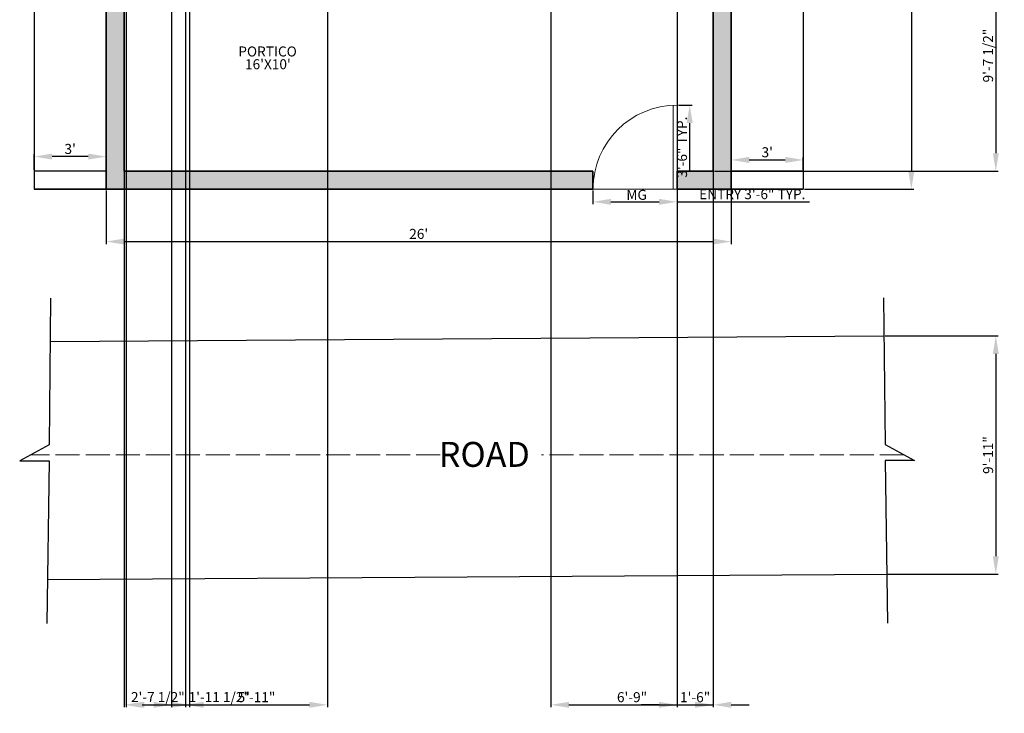
# Model space of a CAD drawing. Units: inches. Extents: x 2265 to 2807, y 1544 to 2401.
# Tile 1 of 9: x 2316 to 2807, y 1544 to 1890. Entities that reach past the tile are written whole.
import ezdxf

# ---------------------------------------------------------------- set-up
doc = ezdxf.new("R2010")
doc.units = ezdxf.units.IN
doc.linetypes.add('ACAD_ISO02W100', pattern=[15, 12, -3])
for name, color, linetype, lineweight in [('A-ANNO-DIMS', 2, 'Continuous', 18), ('A-ANNO-TEXT', 7, 'Continuous', 18), ('A-AREA-IDEN', 7, 'Continuous', 18), ('A-DOOR', 3, 'Continuous', 18), ('A-WALL', 7, 'Continuous', 35), ('A-WALL-PATT', 18, 'Continuous', 13), ('C-PROP', 7, 'Continuous', 25), ('C-ROAD', 8, 'Continuous', 25), ('C-ROAD-CNTR', 8, 'ACAD_ISO02W100', 18)]:
    doc.layers.add(name, color=color, linetype=linetype, lineweight=lineweight)
doc.styles.add('ARIAL', font='times.ttf', dxfattribs={"height": 5})
doc.styles.get("Standard").update_dxf_attribs({"font": 'arial.ttf', "height": 5})
doc.dimstyles.new('ISO-25', dxfattribs={"dimtxt": 5, "dimasz": 9, "dimexe": 1.25, "dimexo": 0.625, "dimtad": 1, "dimlunit": 3, "dimtxsty": 'Standard', "dimcen": 2.5, "dimadec": 0, "dimazin": 0, "dimtfac": 1, "dimtmove": 0, "dimatfit": 3, "dimfxl": 1, "dimarcsym": 0})

# ---------------------------------------------------------------- blocks, each defined once
blk = doc.blocks.new('*D2')
at = {"layer": 'A-ANNO-DIMS', "color": 0, "lineweight": -2, "transparency": 16777216}
for p, q in [((2323.1, 1815.36), (2323.1, 1823.27)), ((2350.1, 1822.02), (2332.1, 1822.02)), ((2359.1, 1815.36), (2359.1, 1823.27))]:
    blk.add_line(p, q, dxfattribs=at)
at = {"layer": 'A-ANNO-DIMS', "color": 0, "lineweight": 100, "transparency": 16777216}
for points in [[(2332.1, 1823.52), (2332.1, 1820.52), (2323.1, 1822.02)], [(2350.1, 1823.52), (2350.1, 1820.52), (2359.1, 1822.02)]]:
    blk.add_solid(points, dxfattribs=at)
at = {"layer": 'Defpoints', "color": 0, "lineweight": 100, "transparency": 16777216}
for p in [(2323.1, 1822.02), (2323.1, 1814.73), (2359.1, 1814.73)]:
    blk.add_point(p, dxfattribs=at)
at = {"layer": 'A-ANNO-DIMS', "color": 0, "transparency": 16777216, "insert": (2341.1, 1825.2), "char_height": 5, "attachment_point": 5}
blk.add_mtext("3'", dxfattribs=at)
blk = doc.blocks.new('*D3')
at = {"layer": 'A-ANNO-DIMS', "color": 0, "lineweight": -2, "transparency": 16777216}
for p, q in [((2671.1, 1815.36), (2671.1, 1821.61)), ((2680.1, 1820.36), (2698.1, 1820.36)), ((2707.1, 1815.36), (2707.1, 1821.61))]:
    blk.add_line(p, q, dxfattribs=at)
at = {"layer": 'A-ANNO-DIMS', "color": 0, "lineweight": 100, "transparency": 16777216}
for points in [[(2680.1, 1821.86), (2680.1, 1818.86), (2671.1, 1820.36)], [(2698.1, 1821.86), (2698.1, 1818.86), (2707.1, 1820.36)]]:
    blk.add_solid(points, dxfattribs=at)
at = {"layer": 'Defpoints', "color": 0, "lineweight": 100, "transparency": 16777216}
for p in [(2707.1, 1820.36), (2671.1, 1814.73), (2707.1, 1814.73)]:
    blk.add_point(p, dxfattribs=at)
at = {"layer": 'A-ANNO-DIMS', "color": 0, "transparency": 16777216, "insert": (2689.1, 1823.54), "char_height": 5, "attachment_point": 5}
blk.add_mtext("3'", dxfattribs=at)
blk = doc.blocks.new('*D4')
at = {"layer": 'A-ANNO-DIMS', "color": 0, "lineweight": -2, "transparency": 16777216}
for p, q in [((2359.1, 1805.11), (2359.1, 1778.33)), ((2671.1, 1805.11), (2671.1, 1778.33)), ((2368.1, 1779.58), (2662.1, 1779.58))]:
    blk.add_line(p, q, dxfattribs=at)
at = {"layer": 'A-ANNO-DIMS', "color": 0, "lineweight": 100, "transparency": 16777216}
for points in [[(2368.1, 1781.08), (2368.1, 1778.08), (2359.1, 1779.58)], [(2662.1, 1781.08), (2662.1, 1778.08), (2671.1, 1779.58)]]:
    blk.add_solid(points, dxfattribs=at)
at = {"layer": 'Defpoints', "color": 0, "lineweight": 100, "transparency": 16777216}
for p in [(2359.1, 1805.73), (2671.1, 1805.73), (2671.1, 1779.58)]:
    blk.add_point(p, dxfattribs=at)
at = {"layer": 'A-ANNO-DIMS', "color": 0, "transparency": 16777216, "insert": (2515.1, 1782.76), "char_height": 5, "attachment_point": 5}
blk.add_mtext("26'", dxfattribs=at)
blk = doc.blocks.new('*D6')
at = {"layer": 'A-ANNO-DIMS', "color": 0, "lineweight": -2, "transparency": 16777216}
for p, q in [((2707.73, 2255.73), (2762.29, 2255.73)), ((2761.04, 2246.73), (2761.04, 1814.73)), ((2707.73, 1805.73), (2762.29, 1805.73))]:
    blk.add_line(p, q, dxfattribs=at)
at = {"layer": 'A-ANNO-DIMS', "color": 0, "lineweight": 100, "transparency": 16777216}
for points in [[(2759.54, 2246.73), (2762.54, 2246.73), (2761.04, 2255.73)], [(2759.54, 1814.73), (2762.54, 1814.73), (2761.04, 1805.73)]]:
    blk.add_solid(points, dxfattribs=at)
at = {"layer": 'Defpoints', "color": 0, "lineweight": 100, "transparency": 16777216}
for p in [(2707.1, 2255.73), (2707.1, 1805.73), (2761.04, 1805.73)]:
    blk.add_point(p, dxfattribs=at)
at = {"layer": 'A-ANNO-DIMS', "color": 0, "transparency": 16777216, "insert": (2757.86, 2030.73), "char_height": 5, "attachment_point": 5, "rotation": 90}
blk.add_mtext('37\'-6"', dxfattribs=at)
blk = doc.blocks.new('ROAD-BREAK')
for p, q in [((15.45, 162.46), (14.64, 89.26)), ((14.64, 89.26), (0, 81.28)), ((0, 81.28), (14.64, 81.28)), ((14.64, 81.28), (13.51, 0))]:
    blk.add_line(p, q)
blk = doc.blocks.new('DOOR-SWING-42IN')
for p, q in [((40, 41.95), (40, 0)), ((42, 0), (0, 0))]:
    blk.add_line(p, q)
blk.add_arc((42, 0), 42, 90, 180)
blk = doc.blocks.new('*D25')
at = {"layer": 'A-ANNO-DIMS', "color": 0, "lineweight": -2, "transparency": 16777216}
for p, q in [((2602.1, 1805.11), (2602.1, 1798.18)), ((2644.1, 1805.11), (2644.1, 1798.18)), ((2611.1, 1799.43), (2635.1, 1799.43)), ((2644.1, 1799.43), (2710.18, 1799.43))]:
    blk.add_line(p, q, dxfattribs=at)
at = {"layer": 'A-ANNO-DIMS', "color": 0, "lineweight": 100, "transparency": 16777216}
for points in [[(2611.1, 1800.93), (2611.1, 1797.93), (2602.1, 1799.43)], [(2635.1, 1800.93), (2635.1, 1797.93), (2644.1, 1799.43)]]:
    blk.add_solid(points, dxfattribs=at)
at = {"layer": 'Defpoints', "color": 0, "lineweight": 100, "transparency": 16777216}
for p in [(2602.1, 1805.73), (2644.1, 1805.73), (2644.1, 1799.43)]:
    blk.add_point(p, dxfattribs=at)
at = {"layer": 'A-ANNO-DIMS', "color": 0, "transparency": 16777216, "insert": (2681.64, 1802.61), "char_height": 5, "attachment_point": 5}
blk.add_mtext('ENTRY 3\'-6" TYP.', dxfattribs=at)
blk = doc.blocks.new('*D26')
at = {"layer": 'A-ANNO-DIMS', "color": 0, "lineweight": -2, "transparency": 16777216}
for p, q in [((2644.73, 1847.73), (2651.65, 1847.73)), ((2650.4, 1814.73), (2650.4, 1838.73)), ((2644.73, 1805.73), (2651.65, 1805.73))]:
    blk.add_line(p, q, dxfattribs=at)
at = {"layer": 'A-ANNO-DIMS', "color": 0, "lineweight": 100, "transparency": 16777216}
for points in [[(2648.9, 1838.73), (2651.9, 1838.73), (2650.4, 1847.73)], [(2648.9, 1814.73), (2651.9, 1814.73), (2650.4, 1805.73)]]:
    blk.add_solid(points, dxfattribs=at)
at = {"layer": 'Defpoints', "color": 0, "lineweight": 100, "transparency": 16777216}
for p in [(2644.1, 1847.73), (2650.4, 1847.73), (2644.1, 1805.73)]:
    blk.add_point(p, dxfattribs=at)
at = {"layer": 'A-ANNO-DIMS', "color": 0, "transparency": 16777216, "insert": (2647.22, 1826.73), "char_height": 5, "attachment_point": 5, "rotation": 90}
blk.add_mtext('3\'-6" TYP.', dxfattribs=at)
blk = doc.blocks.new('*D35')
at = {"layer": 'A-ANNO-DIMS', "color": 0, "lineweight": -2, "transparency": 16777216}
for p, q in [((2581.1, 2123.11), (2581.1, 1546.93)), ((2662.1, 2123.11), (2662.1, 1546.93)), ((2590.1, 1548.18), (2653.1, 1548.18))]:
    blk.add_line(p, q, dxfattribs=at)
at = {"layer": 'A-ANNO-DIMS', "color": 0, "lineweight": 100, "transparency": 16777216}
for points in [[(2590.1, 1549.68), (2590.1, 1546.68), (2581.1, 1548.18)], [(2653.1, 1549.68), (2653.1, 1546.68), (2662.1, 1548.18)]]:
    blk.add_solid(points, dxfattribs=at)
at = {"layer": 'Defpoints', "color": 0, "lineweight": 100, "transparency": 16777216}
for p in [(2581.1, 2123.73), (2662.1, 2123.73), (2662.1, 1548.18)]:
    blk.add_point(p, dxfattribs=at)
at = {"layer": 'A-ANNO-DIMS', "color": 0, "transparency": 16777216, "insert": (2621.6, 1551.36), "char_height": 5, "attachment_point": 5}
blk.add_mtext('6\'-9"', dxfattribs=at)
blk = doc.blocks.new('*D38')
at = {"layer": 'A-ANNO-DIMS', "color": 0, "lineweight": -2, "transparency": 16777216}
for p, q in [((2747.98, 1732.42), (2804.46, 1732.42)), ((2803.21, 1723.42), (2803.21, 1622.43)), ((2749.38, 1613.43), (2804.46, 1613.43))]:
    blk.add_line(p, q, dxfattribs=at)
at = {"layer": 'A-ANNO-DIMS', "color": 0, "lineweight": 100, "transparency": 16777216}
for points in [[(2801.71, 1723.42), (2804.71, 1723.42), (2803.21, 1732.42)], [(2801.71, 1622.43), (2804.71, 1622.43), (2803.21, 1613.43)]]:
    blk.add_solid(points, dxfattribs=at)
at = {"layer": 'Defpoints', "color": 0, "lineweight": 100, "transparency": 16777216}
for p in [(2747.36, 1732.42), (2748.75, 1613.43), (2803.21, 1613.43)]:
    blk.add_point(p, dxfattribs=at)
at = {"layer": 'A-ANNO-DIMS', "color": 0, "transparency": 16777216, "insert": (2800.03, 1672.93), "char_height": 5, "attachment_point": 5, "rotation": 90}
blk.add_mtext('9\'-11"', dxfattribs=at)
blk = doc.blocks.new('*D39')
at = {"layer": 'A-ANNO-DIMS', "color": 0, "lineweight": -2, "transparency": 16777216}
for p, q in [((2644.1, 1929.61), (2644.1, 1546.93)), ((2662.1, 1929.61), (2662.1, 1546.93)), ((2635.1, 1548.18), (2626.1, 1548.18)), ((2644.1, 1548.18), (2662.1, 1548.18)), ((2671.1, 1548.18), (2680.1, 1548.18))]:
    blk.add_line(p, q, dxfattribs=at)
at = {"layer": 'A-ANNO-DIMS', "color": 0, "lineweight": 100, "transparency": 16777216}
for points in [[(2635.1, 1549.68), (2635.1, 1546.68), (2644.1, 1548.18)], [(2671.1, 1549.68), (2671.1, 1546.68), (2662.1, 1548.18)]]:
    blk.add_solid(points, dxfattribs=at)
at = {"layer": 'Defpoints', "color": 0, "lineweight": 100, "transparency": 16777216}
for p in [(2644.1, 1930.23), (2662.1, 1930.23), (2662.1, 1548.18)]:
    blk.add_point(p, dxfattribs=at)
at = {"layer": 'A-ANNO-DIMS', "color": 0, "transparency": 16777216, "insert": (2653.1, 1551.36), "char_height": 5, "attachment_point": 5}
blk.add_mtext('1\'-6"', dxfattribs=at)
blk = doc.blocks.new('*D44')
at = {"layer": 'A-ANNO-DIMS', "color": 0, "lineweight": -2, "transparency": 16777216}
for p, q in [((2369.12, 1940.58), (2369.12, 1546.93)), ((2400.62, 1940.58), (2400.62, 1546.93)), ((2378.12, 1548.18), (2391.62, 1548.18))]:
    blk.add_line(p, q, dxfattribs=at)
at = {"layer": 'A-ANNO-DIMS', "color": 0, "lineweight": 100, "transparency": 16777216}
for points in [[(2378.12, 1549.68), (2378.12, 1546.68), (2369.12, 1548.18)], [(2391.62, 1549.68), (2391.62, 1546.68), (2400.62, 1548.18)]]:
    blk.add_solid(points, dxfattribs=at)
at = {"layer": 'Defpoints', "color": 0, "lineweight": 100, "transparency": 16777216}
for p in [(2369.12, 1941.2), (2400.62, 1941.2), (2400.62, 1548.18)]:
    blk.add_point(p, dxfattribs=at)
at = {"layer": 'A-ANNO-DIMS', "color": 0, "transparency": 16777216, "insert": (2384.87, 1551.4), "char_height": 5, "attachment_point": 5}
blk.add_mtext('2\'-7 1/2"', dxfattribs=at)
blk = doc.blocks.new('*D45')
at = {"layer": 'A-ANNO-DIMS', "color": 0, "lineweight": -2, "transparency": 16777216}
for p, q in [((2391.72, 2088.38), (2391.72, 1546.93)), ((2368.1, 2075.11), (2368.1, 1546.93)), ((2377.1, 1548.18), (2382.72, 1548.18)), ((2391.72, 1548.18), (2430.33, 1548.18))]:
    blk.add_line(p, q, dxfattribs=at)
at = {"layer": 'A-ANNO-DIMS', "color": 0, "lineweight": 100, "transparency": 16777216}
for points in [[(2377.1, 1549.68), (2377.1, 1546.68), (2368.1, 1548.18)], [(2382.72, 1549.68), (2382.72, 1546.68), (2391.72, 1548.18)]]:
    blk.add_solid(points, dxfattribs=at)
at = {"layer": 'Defpoints', "color": 0, "lineweight": 100, "transparency": 16777216}
for p in [(2391.72, 2089), (2368.1, 2075.73), (2391.72, 1548.18)]:
    blk.add_point(p, dxfattribs=at)
at = {"layer": 'A-ANNO-DIMS', "color": 0, "transparency": 16777216, "insert": (2415.53, 1551.4), "char_height": 5, "attachment_point": 5}
blk.add_mtext('1\'-11 1/2"', dxfattribs=at)
blk = doc.blocks.new('*D50')
at = {"layer": 'A-ANNO-DIMS', "color": 0, "lineweight": -2, "transparency": 16777216}
for p, q in [((2398.67, 2169.19), (2398.67, 1546.93)), ((2469.53, 2169.19), (2469.53, 1546.93)), ((2407.67, 1548.18), (2460.53, 1548.18))]:
    blk.add_line(p, q, dxfattribs=at)
at = {"layer": 'A-ANNO-DIMS', "color": 0, "lineweight": 100, "transparency": 16777216}
for points in [[(2407.67, 1549.68), (2407.67, 1546.68), (2398.67, 1548.18)], [(2460.53, 1549.68), (2460.53, 1546.68), (2469.53, 1548.18)]]:
    blk.add_solid(points, dxfattribs=at)
at = {"layer": 'Defpoints', "color": 0, "lineweight": 100, "transparency": 16777216}
for p in [(2398.67, 2169.81), (2469.53, 2169.81), (2469.53, 1548.18)]:
    blk.add_point(p, dxfattribs=at)
at = {"layer": 'A-ANNO-DIMS', "color": 0, "transparency": 16777216, "insert": (2434.1, 1551.36), "char_height": 5, "attachment_point": 5}
blk.add_mtext('5\'-11"', dxfattribs=at)
blk = doc.blocks.new('*D53')
at = {"layer": 'A-ANNO-DIMS', "color": 0, "lineweight": -2, "transparency": 16777216}
for p, q in [((2662.73, 1930.23), (2804.46, 1930.23)), ((2803.21, 1921.23), (2803.21, 1823.73)), ((2662.73, 1814.73), (2804.46, 1814.73))]:
    blk.add_line(p, q, dxfattribs=at)
at = {"layer": 'A-ANNO-DIMS', "color": 0, "lineweight": 100, "transparency": 16777216}
for points in [[(2801.71, 1921.23), (2804.71, 1921.23), (2803.21, 1930.23)], [(2801.71, 1823.73), (2804.71, 1823.73), (2803.21, 1814.73)]]:
    blk.add_solid(points, dxfattribs=at)
at = {"layer": 'Defpoints', "color": 0, "lineweight": 100, "transparency": 16777216}
for p in [(2662.1, 1930.23), (2662.1, 1814.73), (2803.21, 1814.73)]:
    blk.add_point(p, dxfattribs=at)
at = {"layer": 'A-ANNO-DIMS', "color": 0, "transparency": 16777216, "insert": (2800, 1872.48), "char_height": 5, "attachment_point": 5, "rotation": 90}
blk.add_mtext('9\'-7 1/2"', dxfattribs=at)

msp = doc.modelspace()

# ---------------------------------------------------------------- hatches: boundary and pattern name
at = {"layer": 'A-WALL-PATT'}
h = msp.add_hatch(color=256, dxfattribs=at)
h.dxf.hatch_style = 1
h.paths.add_polyline_path([(2416.101, 2255.733), (2359.101, 2255.733), (2359.101, 2205.483), (2368.101, 2205.483), (2368.101, 2246.733), (2416.101, 2246.733)])
h.paths.add_polyline_path([(2528.601, 2255.733), (2452.101, 2255.733), (2452.101, 2246.733), (2487.251, 2246.733), (2500.101, 2246.733), (2500.101, 2168.733), (2504.601, 2168.733), (2504.601, 2170.233), (2525.601, 2170.233), (2525.601, 2174.733), (2504.601, 2174.733), (2504.601, 2246.733), (2528.601, 2246.733)])
h.paths.add_polyline_path([(2603.601, 2255.733), (2552.601, 2255.733), (2552.601, 2246.733), (2576.601, 2246.733), (2576.601, 2174.733), (2555.601, 2174.733), (2555.601, 2170.233), (2576.601, 2170.233), (2576.601, 2123.733), (2581.101, 2123.733), (2581.101, 2246.733), (2603.601, 2246.733)])
h.paths.add_polyline_path([(2671.101, 2255.733), (2639.601, 2255.733), (2639.601, 2246.733), (2662.101, 2246.733), (2662.101, 2083.435), (2671.101, 2083.435)])
h.paths.add_polyline_path([(2671.101, 2035.435), (2662.101, 2035.435), (2662.101, 1939.233), (2644.101, 1939.233), (2644.101, 1930.233), (2662.101, 1930.233), (2662.101, 1814.733), (2644.101, 1814.733), (2644.101, 1805.733), (2671.101, 1805.733)])
h.paths.add_polyline_path([(2368.101, 1930.233), (2511.351, 1930.233), (2511.351, 1939.233), (2468.601, 1939.233), (2468.601, 2032.233), (2464.101, 2032.233), (2464.101, 1939.233), (2368.101, 1939.233), (2368.101, 1995.884), (2359.101, 1995.884), (2359.101, 1805.733), (2602.101, 1805.733), (2602.101, 1814.733), (2368.101, 1814.733)])
h.paths.add_polyline_path([(2368.101, 2071.233), (2464.101, 2071.233), (2464.101, 2062.233), (2468.601, 2062.233), (2468.601, 2123.733), (2504.601, 2123.733), (2504.601, 2132.733), (2500.101, 2132.733), (2500.101, 2128.233), (2455.101, 2128.233), (2455.101, 2123.733), (2464.101, 2123.733), (2464.101, 2075.733), (2368.101, 2075.733), (2368.101, 2087.733), (2359.101, 2087.733), (2359.101, 2031.884), (2368.101, 2031.884)])
h.paths.add_polyline_path([(2368.101, 2169.483), (2359.101, 2169.483), (2359.101, 2111.733), (2368.101, 2111.733), (2368.101, 2123.733), (2425.101, 2123.733), (2425.101, 2128.233), (2368.101, 2128.233)])

# ---------------------------------------------------------------- linework, layer by layer
at = {"layer": 'A-DOOR'}
msp.add_line((2644.101, 1847.733), (2644.101, 1805.733), dxfattribs=at)
at = {"layer": 'A-WALL'}
for p, q in [((2359.101, 1805.733), (2359.101, 2255.733)), ((2671.101, 2255.733), (2671.101, 1805.733)), ((2368.101, 1814.733), (2368.101, 1930.233)), ((2662.101, 1930.233), (2662.101, 1814.733)), ((2602.101, 1814.733), (2368.101, 1814.733)), ((2602.101, 1814.733), (2602.101, 1805.733)), ((2662.101, 1814.733), (2644.101, 1814.733)), ((2644.101, 1814.733), (2644.101, 1805.733)), ((2602.101, 1805.733), (2323.101, 1805.733)), ((2707.101, 1805.733), (2644.101, 1805.733))]:
    msp.add_line(p, q, dxfattribs=at)
at = {"layer": 'C-PROP'}
for p, q in [((2323.101, 2255.733), (2323.101, 1805.733)), ((2707.101, 2255.733), (2707.101, 1805.733)), ((2359.101, 1814.733), (2323.101, 1814.733)), ((2707.101, 1814.733), (2671.101, 1814.733))]:
    msp.add_line(p, q, dxfattribs=at)
at = {"layer": 'C-ROAD'}
for p, q in [((2331.35, 1729.707), (2747.36, 1732.423)), ((2329.714, 1610.743), (2748.751, 1613.43))]:
    msp.add_line(p, q, dxfattribs=at)
at = {"layer": 'C-ROAD-CNTR'}
for p, q in [((2525.837, 1673.105), (2321.457, 1673.105)), ((2757.366, 1673.105), (2576.325, 1673.105))]:
    msp.add_line(p, q, dxfattribs=at)

# ---------------------------------------------------------------- block references
at = {"layer": 'A-DOOR'}
msp.add_blockref('DOOR-SWING-42IN', (2602.101, 1805.733), dxfattribs=at)
at = {"layer": 'C-ROAD'}
msp.add_blockref('ROAD-BREAK', (2315.899, 1588.795), dxfattribs=at)
at = {"layer": 'C-ROAD', "extrusion": (0, 0, -1), "zscale": -1}
msp.add_blockref('ROAD-BREAK', (-2762.6, 1588.972), dxfattribs=at)

# ---------------------------------------------------------------- texts
at = {"layer": 'A-ANNO-TEXT', "style": 'ARIAL'}
msp.add_text('MG', height=5, dxfattribs=at).set_placement((2618.769, 1800.419))
at = {"layer": 'A-ANNO-TEXT'}
msp.add_text('ROAD', height=12.4694, dxfattribs=at).set_placement((2525.129, 1667.041))
at = {"layer": 'A-AREA-IDEN', "style": 'ARIAL'}
for s, p in [('PORTICO', (2425.035, 1872.032)), ("16'X10'", (2428.385, 1865.671))]:
    msp.add_text(s, height=5, dxfattribs=at).set_placement(p)

# ---------------------------------------------------------------- dimensions: what is measured, and where the dimension line sits
at = {"layer": 'A-ANNO-DIMS'}
for base, p1, p2, override, picture, middle in [((2761.041, 1805.733), (2707.101, 2255.733), (2707.101, 1805.733), {"dimclrd": 0, "dimclre": 0, "dimclrt": 0}, '*D6', (2757.861, 2030.733)), ((2803.21, 1814.733), (2662.101, 1930.233), (2662.101, 1814.733), {"dimdec": 1, "dimlfac": 1, "dimrnd": 0, "dimzin": 1, "dimdsep": 46, "dimlunit": 4, "dimfrac": 2}, '*D53', (2800, 1872.483)), ((2803.21, 1613.43), (2747.36, 1732.423), (2748.751, 1613.43), {"dimdec": 1, "dimlfac": 1, "dimrnd": 0, "dimzin": 1, "dimdsep": 46, "dimlunit": 4, "dimfrac": 2}, '*D38', (2800.032, 1672.927))]:
    dim = msp.add_linear_dim(base=base, p1=p1, p2=p2, angle=90, dimstyle='ISO-25', override=override, dxfattribs=at)
    dim.commit()
    dim.dimension.update_dxf_attribs({"geometry": picture, "text_midpoint": middle})
for base, p1, p2, override, picture, middle in [((2469.534, 1548.185), (2398.668, 2169.812), (2469.534, 2169.812), {"dimdec": 1, "dimlfac": 1, "dimrnd": 0, "dimzin": 1, "dimdsep": 46, "dimlunit": 4, "dimfrac": 2}, '*D50', (2434.101, 1551.363)), ((2662.101, 1548.185), (2581.101, 2123.733), (2662.101, 2123.733), {"dimdec": 1, "dimlfac": 1, "dimrnd": 0, "dimzin": 1, "dimdsep": 46, "dimlunit": 4, "dimfrac": 2}, '*D35', (2621.601, 1551.363)), ((2391.723, 1548.185), (2368.101, 2075.733), (2391.723, 2089.003), {"dimdec": 1, "dimlfac": 1, "dimrnd": 0, "dimzin": 1, "dimdsep": 46, "dimlunit": 4, "dimfrac": 2}, '*D45', (2415.526, 1551.395)), ((2400.615, 1548.185), (2369.119, 1941.202), (2400.615, 1941.202), {"dimdec": 1, "dimlfac": 1, "dimrnd": 0, "dimzin": 1, "dimdsep": 46, "dimlunit": 4, "dimfrac": 2}, '*D44', (2384.867, 1551.395)), ((2662.101, 1548.185), (2644.101, 1930.233), (2662.101, 1930.233), {"dimdec": 1, "dimlfac": 1, "dimrnd": 0, "dimzin": 1, "dimdsep": 46, "dimlunit": 4, "dimfrac": 2}, '*D39', (2653.101, 1551.363)), ((2323.101, 1822.018), (2359.101, 1814.733), (2323.101, 1814.733), {"dimclrd": 0, "dimclre": 0, "dimclrt": 0}, '*D2', (2341.101, 1825.198)), ((2707.101, 1820.356), (2671.101, 1814.733), (2707.101, 1814.733), {"dimclrd": 0, "dimclre": 0, "dimclrt": 0}, '*D3', (2689.101, 1823.536)), ((2671.101, 1779.58), (2359.101, 1805.733), (2671.101, 1805.733), {"dimclrd": 0, "dimclre": 0, "dimclrt": 0}, '*D4', (2515.101, 1782.758))]:
    dim = msp.add_linear_dim(base=base, p1=p1, p2=p2, dimstyle='ISO-25', override=override, dxfattribs=at)
    dim.commit()
    dim.dimension.update_dxf_attribs({"geometry": picture, "text_midpoint": middle})
dim = msp.add_linear_dim(base=(2650.401, 1847.733), p1=(2644.101, 1805.733), p2=(2644.101, 1847.733), angle=90, text='<> TYP.', dimstyle='ISO-25', override={"dimdec": 1, "dimlfac": 1, "dimrnd": 0, "dimzin": 1, "dimdsep": 46, "dimlunit": 4, "dimfrac": 2}, dxfattribs=at)
dim.commit()
dim.dimension.update_dxf_attribs({"geometry": '*D26', "text_midpoint": (2647.222, 1826.733)})
dim = msp.add_linear_dim(base=(2644.101, 1799.433), p1=(2602.101, 1805.733), p2=(2644.101, 1805.733), text='ENTRY <> TYP.', dimstyle='ISO-25', override={"dimdec": 1, "dimlfac": 1, "dimrnd": 0, "dimzin": 1, "dimdsep": 46, "dimlunit": 4, "dimfrac": 2}, dxfattribs=at)
dim.commit()
dim.dimension.update_dxf_attribs({"geometry": '*D25', "text_midpoint": (2681.641, 1802.613)})

doc.saveas('drawing.dxf')
